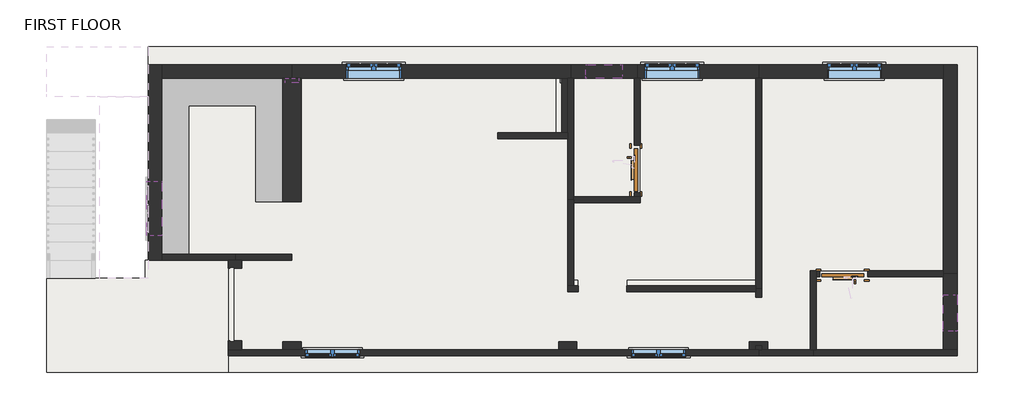
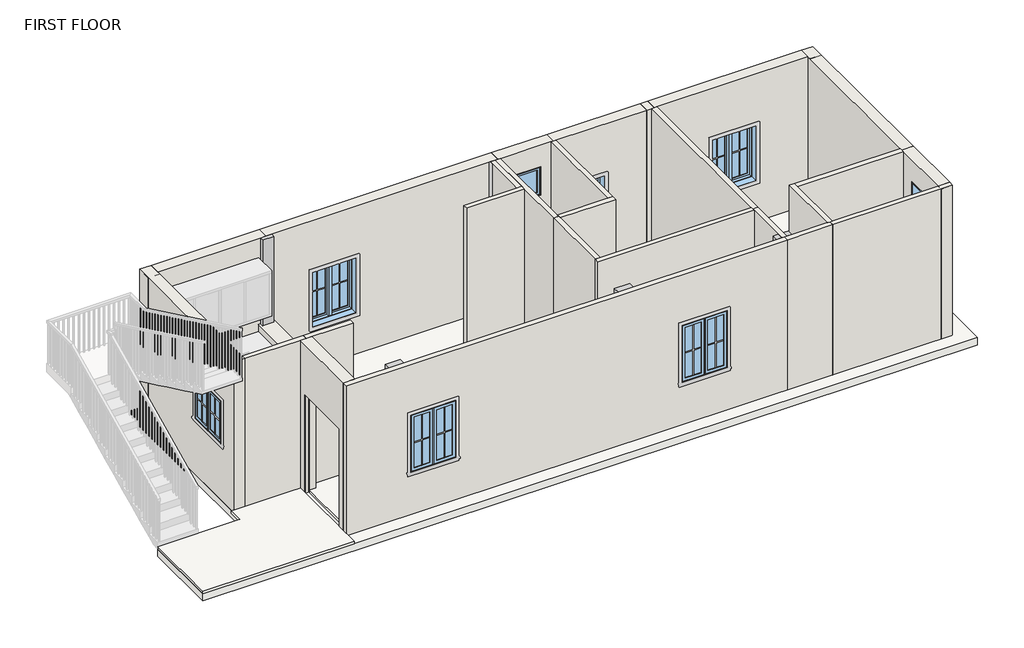
# One storey, part 1 of 3: 26 walls, 8 windows, 6 columns, 4 slabs, 2 doors.
"""IFC4 building model written with IfcOpenShell, lengths in millimetres."""

from ifc_helpers import new_model, si_unit, frame, origin, place, context, project, spatial, polyline, outline, extrude, faceted_brep, transform, mapped, element, save
from components import apartment_toilet_door_15897_d3_toilet_d7560075, apartment_toilet_door_15897_d3_toilet_03746f18, window_80340324, window_casement_double_w1_d341e8ac, window_casement_double_w1_80f1179f, window_casement_double_w1_2_90de19e9

model = new_model("IFC4")

# Units and contexts
model_context = context("Model", 3, world=origin())
ifc_project = project(units=[si_unit("LENGTHUNIT", "METRE", prefix="MILLI")], contexts=[model_context])

# Site, building, storey
site = spatial("IfcSite", under=ifc_project)
building = spatial("IfcBuilding", under=site)
storey = spatial("IfcBuildingStorey", under=building, Name="FIRST FLOOR", Elevation=3200.4)

# Columns
placement = place(None, origin())
element("IfcColumn", 1, ObjectType="Rectangular Column : 9\" X 12\"", at=placement, inside=storey, context=model_context, shape_type="SweptSolid", body=[
    extrude(outline(polyline([(-2166.0591227, 4797.7642852), (-2394.6591227, 4797.7642852), (-2394.6591227, 4873.9642852), (-2280.3591227, 4873.9642852), (-2166.0591227, 4873.9642852), (-2166.0591227, 4797.7642852)])), frame((0.0, 0.0, 4572.0), z_axis=(0.0, 0.0, 1.0), x_axis=(1.0, 0.0, 0.0)), (0.0, 0.0, 1.0), 1828.8),
])
element("IfcColumn", 2, ObjectType="Rectangular Column : 9\" X 12\"", at=placement, inside=storey, context=model_context, shape_type="Brep", body=[
    faceted_brep([(-4693.3591227, 5102.5642852, 3200.4), (-4464.7591227, 5102.5642852, 3200.4), (-4464.7591227, 4873.9642852, 3200.4), (-4464.7591227, 4797.7642852, 3200.4), (-4693.3591227, 4797.7642852, 3200.4), (-4693.3591227, 5102.5642852, 6400.8), (-4464.7591227, 5102.5642852, 6400.8), (-4464.7591227, 4873.9642852, 6400.8), (-4464.7591227, 4797.7642852, 6400.8), (-4693.3591227, 4797.7642852, 6400.8)], [[[0, 1, 2, 3, 4]], [[5, 6, 1, 0]], [[6, 7, 8, 3, 2, 1]], [[8, 9, 4, 3]], [[9, 5, 0, 4]], [[5, 9, 8, 7, 6]]]),
])
element("IfcColumn", 3, ObjectType="Rectangular Column : 9\" X 12\"", at=placement, inside=storey, context=model_context, shape_type="Brep", body=[
    faceted_brep([(5390.4408773, 454.3642852, 3200.4), (5695.2408773, 454.3642852, 3200.4), (5695.2408773, 327.3642852, 3200.4), (5593.6408773, 327.3642852, 3200.4), (5593.6408773, 390.8642852, 3200.4), (5492.0408773, 390.8642852, 3200.4), (5492.0408773, 327.3642852, 3200.4), (5390.4408773, 327.3642852, 3200.4), (5695.2408773, 454.3642852, 6400.8), (5695.2408773, 327.3642852, 6400.8), (5390.4408773, 454.3642852, 6400.8), (5390.4408773, 327.3642852, 6400.8), (5492.0408773, 454.3642852, 6400.8), (5492.0408773, 454.3642852, 5334.0), (5593.6408773, 454.3642852, 5334.0), (5593.6408773, 454.3642852, 6400.8), (5593.6408773, 327.3642852, 6400.8), (5593.6408773, 390.8642852, 5334.0), (5492.0408773, 390.8642852, 5334.0), (5492.0408773, 327.3642852, 6400.8)], [[[0, 1, 2, 3, 4, 5, 6, 7]], [[1, 8, 9, 2]], [[10, 0, 7, 11]], [[1, 0, 10, 12, 13, 14, 15, 8]], [[8, 15, 16, 9]], [[17, 4, 3, 16, 15, 14]], [[5, 18, 13, 12, 19, 6]], [[4, 17, 18, 5]], [[18, 17, 14, 13]], [[7, 6, 19, 11]], [[12, 10, 11, 19]], [[3, 2, 9, 16]]]),
])
element("IfcColumn", 4, ObjectType="Rectangular Column : 9\" X 12\"", at=placement, inside=storey, context=model_context, shape_type="SweptSolid", body=[
    extrude(outline(polyline([(2190.0408773, 454.3642852), (2494.8408773, 454.3642852), (2494.8408773, 327.3642852), (2190.0408773, 327.3642852), (2190.0408773, 454.3642852)])), frame((0.0, 0.0, 3200.4), z_axis=(0.0, 0.0, 1.0), x_axis=(1.0, 0.0, 0.0)), (0.0, 0.0, 1.0), 3200.4),
])
element("IfcColumn", 5, ObjectType="Rectangular Column : 9\" X 12\"", at=placement, inside=storey, context=model_context, shape_type="SweptSolid", body=[
    extrude(outline(polyline([(-2432.7591227, 454.3642852), (-2127.9591227, 454.3642852), (-2127.9591227, 327.3642852), (-2432.7591227, 327.3642852), (-2432.7591227, 454.3642852)])), frame((0.0, 0.0, 3200.4), z_axis=(0.0, 0.0, 1.0), x_axis=(1.0, 0.0, 0.0)), (0.0, 0.0, 1.0), 3200.4),
])
element("IfcColumn", 6, ObjectType="Rectangular Column : 9\" X 12\"", at=placement, inside=storey, context=model_context, shape_type="Brep", body=[
    faceted_brep([(-4693.3591227, 2130.7642852, 3200.4), (-4464.7591227, 2130.7642852, 3200.4), (-4464.7591227, 1927.5642852, 3200.4), (-4464.7591227, 1825.9642852, 3200.4), (-4693.3591227, 1825.9642852, 3200.4), (-4693.3591227, 2130.7642852, 6400.8), (-4464.7591227, 2130.7642852, 6400.8), (-4464.7591227, 1927.5642852, 6400.8), (-4464.7591227, 1825.9642852, 6400.8), (-4693.3591227, 1825.9642852, 6400.8)], [[[0, 1, 2, 3, 4]], [[5, 6, 1, 0]], [[6, 7, 8, 3, 2, 1]], [[8, 9, 4, 3]], [[9, 5, 0, 4]], [[5, 9, 8, 7, 6]]]),
])

# Doors
apartment_toilet_door_15897_d3_toilet_shape = apartment_toilet_door_15897_d3_toilet_d7560075(model_context)
element("IfcDoor", 7, ObjectType="Apartment_Toilet_Door_15897 : D3 TOILET", at=placement, inside=storey, context=model_context, shape_type="MappedRepresentation", body=[
    mapped(apartment_toilet_door_15897_d3_toilet_shape, transform((6952.5408773, 1597.3642852, 3200.4), x_axis=(-1.0, 0.0, 0.0), y_axis=(0.0, -1.0, 0.0), z_axis=(0.0, 0.0, 1.0))),
])
apartment_toilet_door_15897_d3_toilet_2_shape = apartment_toilet_door_15897_d3_toilet_03746f18(model_context)
element("IfcDoor", 8, ObjectType="Apartment_Toilet_Door_15897 : D3 TOILET", at=placement, inside=storey, context=model_context, shape_type="MappedRepresentation", body=[
    mapped(apartment_toilet_door_15897_d3_toilet_2_shape, transform((3510.8408773, 3337.2642852, 3200.4), x_axis=(0.0, -1.0, 0.0), y_axis=(1.0, 0.0, 0.0), z_axis=(0.0, 0.0, 1.0))),
])

# Slabs
element("IfcSlab", 9, ObjectType="6\" SLAB", at=placement, inside=storey, context=model_context, shape_type="SweptSolid", body=[
    extrude(outline(polyline([(9213.1408773, 5407.3642852), (9213.1408773, 113.4304234), (9213.1408773, -53.6357148), (-6395.1591227, -53.6357148), (-6395.1591227, 1521.1642852), (-4693.3591227, 1521.1642852), (-4693.3591227, 5407.3642852), (9213.1408773, 5407.3642852)])), frame((0.0, 0.0, 3048.0), z_axis=(0.0, 0.0, 1.0), x_axis=(1.0, 0.0, 0.0)), (0.0, 0.0, 1.0), 152.4),
])
element("IfcSlab", 10, ObjectType="FLOORING", at=placement, inside=storey, context=model_context, shape_type="SweptSolid", body=[
    extrude(outline(polyline([(-4464.7591227, 1927.5642852), (-4464.7591227, 4873.9642852), (-2432.7591227, 4873.9642852), (-2432.7591227, 2803.8642852), (-2127.9591227, 2803.8642852), (-2127.9591227, 4873.9642852), (2139.2408773, 4873.9642852), (2139.2408773, 3959.5642852), (1174.0408773, 3959.5642852), (1174.0408773, 3857.9642852), (2342.4408773, 3857.9642852), (2342.4408773, 1394.1642852), (2520.2408773, 1394.1642852), (2520.2408773, 1495.7642852), (2444.0408773, 1495.7642852), (2444.0408773, 2791.1642852), (3561.6408773, 2791.1642852), (3561.6408773, 4873.9642852), (5492.0408773, 4873.9642852), (5492.0408773, 1495.7642852), (3409.2408773, 1495.7642852), (3333.0408773, 1495.7642852), (3333.0408773, 1394.1642852), (5492.0408773, 1394.1642852), (5492.0408773, 1203.6642852), (5593.6408773, 1203.6642852), (5593.6408773, 4873.9642852), (8641.6408773, 4873.9642852), (8641.6408773, 1648.1642852), (6406.4408773, 1648.1642852), (6406.4408773, 327.3642852), (5593.6408773, 327.3642852), (5593.6408773, 390.8642852), (5492.0408773, 390.8642852), (5492.0408773, 327.3642852), (-3118.5591227, 327.3642852), (-3118.5591227, 397.6642852), (-3250.1591227, 397.6642852), (-3250.1591227, 1769.2642852), (-3118.5591227, 1769.2642852), (-3118.5591227, 1825.9642852), (-2280.3591227, 1825.9642852), (-2280.3591227, 1927.5642852), (-4464.7591227, 1927.5642852)])), frame((0.0, 0.0, 3200.4), z_axis=(0.0, 0.0, 1.0), x_axis=(1.0, 0.0, 0.0)), (0.0, 0.0, 1.0), 50.8),
])
element("IfcSlab", 11, ObjectType="FLOORING OPEN AREA", at=placement, inside=storey, context=model_context, shape_type="SweptSolid", body=[
    extrude(outline(polyline([(-3347.1591227, -53.6357148), (-6395.1591227, -53.6357148), (-6395.1591227, 1521.1642852), (-4744.1591227, 1521.1642852), (-4744.1591227, 1825.9642852), (-3347.1591227, 1825.9642852), (-3347.1591227, -53.6357148)])), frame((0.0, 0.0, 3200.4), z_axis=(0.0, 0.0, 1.0), x_axis=(1.0, 0.0, 0.0)), (0.0, 0.0, 1.0), 50.8),
])
element("IfcSlab", 12, ObjectType="FLOORING TOILET", at=placement, inside=storey, context=model_context, shape_type="SweptSolid", body=[
    extrude(outline(polyline([(7371.5408773, 1546.5642852), (8641.6408773, 1546.5642852), (8641.6408773, 327.3642852), (6508.0408773, 327.3642852), (6508.0408773, 1546.5642852), (6571.5408773, 1546.5642852), (6571.5408773, 1648.1642852), (7371.5408773, 1648.1642852), (7371.5408773, 1546.5642852)])), frame((0.0, 0.0, 3200.4), z_axis=(0.0, 0.0, 1.0), x_axis=(1.0, 0.0, 0.0)), (0.0, 0.0, 1.0), 50.8),
    extrude(outline(polyline([(3460.0408773, 4873.9642852), (3460.0408773, 3756.2642852), (3561.6408773, 3756.2642852), (3561.6408773, 2956.2642852), (3460.0408773, 2956.2642852), (3460.0408773, 2892.7642852), (2444.0408773, 2892.7642852), (2444.0408773, 4873.9642852), (3460.0408773, 4873.9642852)])), frame((0.0, 0.0, 3200.4), z_axis=(0.0, 0.0, 1.0), x_axis=(1.0, 0.0, 0.0)), (0.0, 0.0, 1.0), 50.8),
])

# Walls
element("IfcWall", 13, at=placement, inside=storey, context=model_context, shape_type="Brep", body=[
    faceted_brep([(-2432.7591227, 4873.9642852, 3200.4), (-2432.7591227, 2803.8642852, 3200.4), (-2432.7591227, 2803.8642852, 4572.0), (-2432.7591227, 4873.9642852, 4572.0), (-2127.9591227, 4873.9642852, 3200.4), (-2127.9591227, 4873.9642852, 4572.0), (-2127.9591227, 2803.8642852, 4572.0), (-2127.9591227, 2803.8642852, 3200.4), (-2280.3591227, 4873.9642852, 3200.4), (-2166.0591227, 4873.9642852, 4572.0), (-2280.3591227, 4873.9642852, 4572.0), (-2394.6591227, 4873.9642852, 4572.0)], [[[0, 1, 2, 3]], [[4, 5, 6, 7]], [[1, 0, 8, 4, 7]], [[2, 1, 7, 6]], [[3, 2, 6, 5, 9, 10, 11]], [[0, 3, 11, 10, 9, 5, 4, 8]]]),
])
element("IfcWall", 14, ObjectType="4\" WALL", at=placement, inside=storey, context=model_context, shape_type="Brep", body=[
    faceted_brep([(8870.2408773, 327.3642852, 3200.4), (8641.6408773, 327.3642852, 3200.4), (6508.0408773, 327.3642852, 3200.4), (6457.2408773, 327.3642852, 3200.4), (6457.2408773, 327.3642852, 6400.8), (6508.0408773, 327.3642852, 6400.8), (8641.6408773, 327.3642852, 6400.8), (8870.2408773, 327.3642852, 6400.8), (8870.2408773, 225.7642852, 3200.4), (8870.2408773, 225.7642852, 6400.8), (6457.2408773, 225.7642852, 6400.8), (6457.2408773, 225.7642852, 3200.4)], [[[0, 1, 2, 3, 4, 5, 6, 7]], [[8, 9, 10, 11]], [[3, 2, 1, 0, 8, 11]], [[4, 3, 11, 10]], [[7, 6, 5, 4, 10, 9]], [[0, 7, 9, 8]]]),
])
element("IfcWall", 15, ObjectType="4\" WALL", at=placement, inside=storey, context=model_context, shape_type="Brep", body=[
    faceted_brep([(-2280.3591227, 1927.5642852, 3200.4), (-3232.8591227, 1927.5642852, 3200.4), (-3232.8591227, 1927.5642852, 6400.8), (-2280.3591227, 1927.5642852, 6400.8), (-2280.3591227, 1825.9642852, 3200.4), (-2280.3591227, 1825.9642852, 6400.8), (-3118.5591227, 1825.9642852, 6400.8), (-3232.8591227, 1825.9642852, 6400.8), (-3232.8591227, 1825.9642852, 3200.4), (-3118.5591227, 1825.9642852, 3200.4)], [[[0, 1, 2, 3]], [[4, 5, 6, 7, 8, 9]], [[1, 0, 4, 9, 8]], [[2, 1, 8, 7]], [[3, 2, 7, 6, 5]], [[0, 3, 5, 4]]]),
])
element("IfcWall", 16, ObjectType="4\" WALL", at=placement, inside=storey, context=model_context, shape_type="Brep", body=[
    faceted_brep([(5593.6408773, 1343.3642852, 3200.4), (5593.6408773, 1343.3642852, 6400.8), (5593.6408773, 454.3642852, 6400.8), (5593.6408773, 327.3642852, 6400.8), (5593.6408773, 327.3642852, 3200.4), (5593.6408773, 390.8642852, 3200.4), (5593.6408773, 390.8642852, 5334.0), (5593.6408773, 454.3642852, 5334.0), (5593.6408773, 1203.6642852, 5334.0), (5593.6408773, 1203.6642852, 3200.4), (5492.0408773, 1343.3642852, 6400.8), (5492.0408773, 1343.3642852, 3200.4), (5492.0408773, 1292.5642852, 3200.4), (5492.0408773, 1203.6642852, 3200.4), (5492.0408773, 1203.6642852, 5334.0), (5492.0408773, 454.3642852, 5334.0), (5492.0408773, 390.8642852, 5334.0), (5492.0408773, 390.8642852, 3200.4), (5492.0408773, 327.3642852, 3200.4), (5492.0408773, 327.3642852, 6400.8), (5492.0408773, 454.3642852, 6400.8), (5492.0408773, 1292.5642852, 6400.8), (5542.8408773, 327.3642852, 3200.4), (5542.8408773, 327.3642852, 6400.8)], [[[0, 1, 2, 3, 4, 5, 6, 7, 8, 9]], [[10, 11, 12, 13, 14, 15, 16, 17, 18, 19, 20, 21]], [[11, 0, 9, 13, 12]], [[4, 22, 18, 17, 5]], [[1, 0, 11, 10]], [[3, 2, 1, 10, 21, 20, 19, 23]], [[4, 3, 23, 19, 18, 22]], [[16, 6, 5, 17]], [[6, 16, 15, 14, 8, 7]], [[8, 14, 13, 9]]]),
])
element("IfcWall", 17, ObjectType="4\" WALL", at=placement, inside=storey, context=model_context, shape_type="Brep", body=[
    faceted_brep([(5492.0408773, 1394.1642852, 3200.4), (3333.0408773, 1394.1642852, 3200.4), (3333.0408773, 1394.1642852, 5334.0), (2520.2408773, 1394.1642852, 5334.0), (2520.2408773, 1394.1642852, 3200.4), (2444.0408773, 1394.1642852, 3200.4), (2342.4408773, 1394.1642852, 3200.4), (2342.4408773, 1394.1642852, 6400.8), (2444.0408773, 1394.1642852, 6400.8), (5492.0408773, 1394.1642852, 6400.8), (3333.0408773, 1292.5642852, 5334.0), (3333.0408773, 1292.5642852, 3200.4), (5492.0408773, 1292.5642852, 3200.4), (5492.0408773, 1292.5642852, 6400.8), (2342.4408773, 1292.5642852, 6400.8), (2342.4408773, 1292.5642852, 3200.4), (2520.2408773, 1292.5642852, 3200.4), (2520.2408773, 1292.5642852, 5334.0), (5492.0408773, 1343.3642852, 3200.4), (5492.0408773, 1343.3642852, 6400.8)], [[[0, 1, 2, 3, 4, 5, 6, 7, 8, 9]], [[10, 11, 12, 13, 14, 15, 16, 17]], [[16, 15, 6, 5, 4]], [[12, 11, 1, 0, 18]], [[9, 8, 7, 14, 13, 19]], [[0, 9, 19, 13, 12, 18]], [[7, 6, 15, 14]], [[2, 1, 11, 10]], [[3, 2, 10, 17]], [[4, 3, 17, 16]]]),
])
element("IfcWall", 18, ObjectType="4\" WALL", at=placement, inside=storey, context=model_context, shape_type="Brep", body=[
    faceted_brep([(2444.0408773, 1394.1642852, 3200.4), (2444.0408773, 2791.1642852, 3200.4), (2444.0408773, 2841.9642852, 3200.4), (2444.0408773, 2841.9642852, 6400.8), (2444.0408773, 2791.1642852, 6400.8), (2444.0408773, 1394.1642852, 6400.8), (2342.4408773, 1394.1642852, 3200.4), (2342.4408773, 1394.1642852, 6400.8), (2342.4408773, 2841.9642852, 6400.8), (2342.4408773, 2841.9642852, 3200.4)], [[[0, 1, 2, 3, 4, 5]], [[6, 7, 8, 9]], [[2, 1, 0, 6, 9]], [[3, 2, 9, 8]], [[5, 4, 3, 8, 7]], [[0, 5, 7, 6]]]),
])
element("IfcWall", 19, ObjectType="4\" WALL", at=placement, inside=storey, context=model_context, shape_type="Brep", body=[
    faceted_brep([(2342.4408773, 3959.5642852, 3200.4), (2240.8408773, 3959.5642852, 3200.4), (1174.0408773, 3959.5642852, 3200.4), (1174.0408773, 3959.5642852, 6400.8), (2240.8408773, 3959.5642852, 6400.8), (2342.4408773, 3959.5642852, 6400.8), (2342.4408773, 3857.9642852, 3200.4), (2342.4408773, 3857.9642852, 6400.8), (1174.0408773, 3857.9642852, 6400.8), (1174.0408773, 3857.9642852, 3200.4)], [[[0, 1, 2, 3, 4, 5]], [[6, 7, 8, 9]], [[2, 1, 0, 6, 9]], [[3, 2, 9, 8]], [[5, 4, 3, 8, 7]], [[0, 5, 7, 6]]]),
])
element("IfcWall", 20, ObjectType="4\" WALL", at=placement, inside=storey, context=model_context, shape_type="Brep", body=[
    faceted_brep([(6508.0408773, 327.3642852, 3200.4), (6508.0408773, 1546.5642852, 3200.4), (6508.0408773, 1648.1642852, 3200.4), (6508.0408773, 1648.1642852, 6400.8), (6508.0408773, 1546.5642852, 6400.8), (6508.0408773, 327.3642852, 6400.8), (6406.4408773, 327.3642852, 3200.4), (6406.4408773, 327.3642852, 6400.8), (6406.4408773, 1648.1642852, 6400.8), (6406.4408773, 1648.1642852, 3200.4), (6457.2408773, 327.3642852, 3200.4), (6457.2408773, 327.3642852, 6400.8)], [[[0, 1, 2, 3, 4, 5]], [[6, 7, 8, 9]], [[2, 1, 0, 10, 6, 9]], [[5, 4, 3, 8, 7, 11]], [[0, 5, 11, 7, 6, 10]], [[3, 2, 9, 8]]]),
])
element("IfcWall", 21, ObjectType="4\" WALL", at=placement, inside=storey, context=model_context, shape_type="Brep", body=[
    faceted_brep([(6508.0408773, 1546.5642852, 3200.4), (6571.5408773, 1546.5642852, 3200.4), (6571.5408773, 1546.5642852, 5334.0), (7371.5408773, 1546.5642852, 5334.0), (7371.5408773, 1546.5642852, 3200.4), (8641.6408773, 1546.5642852, 3200.4), (8641.6408773, 1546.5642852, 6400.8), (6508.0408773, 1546.5642852, 6400.8), (6571.5408773, 1648.1642852, 5334.0), (6571.5408773, 1648.1642852, 3200.4), (6508.0408773, 1648.1642852, 3200.4), (6508.0408773, 1648.1642852, 6400.8), (8641.6408773, 1648.1642852, 6400.8), (8641.6408773, 1648.1642852, 3200.4), (7371.5408773, 1648.1642852, 3200.4), (7371.5408773, 1648.1642852, 5334.0), (8641.6408773, 1597.3642852, 3200.4), (8641.6408773, 1597.3642852, 6400.8)], [[[0, 1, 2, 3, 4, 5, 6, 7]], [[8, 9, 10, 11, 12, 13, 14, 15]], [[14, 13, 16, 5, 4]], [[10, 9, 1, 0]], [[7, 6, 17, 12, 11]], [[0, 7, 11, 10]], [[6, 5, 16, 13, 12, 17]], [[2, 1, 9, 8]], [[3, 2, 8, 15]], [[4, 3, 15, 14]]]),
])
element("IfcWall", 22, ObjectType="4\" WALL", at=placement, inside=storey, context=model_context, shape_type="Brep", body=[
    faceted_brep([(2444.0408773, 2791.1642852, 3200.4), (3561.6408773, 2791.1642852, 3200.4), (3561.6408773, 2791.1642852, 6400.8), (2444.0408773, 2791.1642852, 6400.8), (2444.0408773, 2892.7642852, 3200.4), (2444.0408773, 2892.7642852, 6400.8), (3460.0408773, 2892.7642852, 6400.8), (3561.6408773, 2892.7642852, 6400.8), (3561.6408773, 2892.7642852, 3200.4), (3460.0408773, 2892.7642852, 3200.4), (2444.0408773, 2841.9642852, 3200.4), (2444.0408773, 2841.9642852, 6400.8)], [[[0, 1, 2, 3]], [[4, 5, 6, 7, 8, 9]], [[1, 0, 10, 4, 9, 8]], [[3, 2, 7, 6, 5, 11]], [[0, 3, 11, 5, 4, 10]], [[2, 1, 8, 7]]]),
])
element("IfcWall", 23, ObjectType="4\" WALL", at=placement, inside=storey, context=model_context, shape_type="Brep", body=[
    faceted_brep([(3561.6408773, 2892.7642852, 3200.4), (3561.6408773, 2956.2642852, 3200.4), (3561.6408773, 2956.2642852, 5334.0), (3561.6408773, 3756.2642852, 5334.0), (3561.6408773, 3756.2642852, 3200.4), (3561.6408773, 4873.9642852, 3200.4), (3561.6408773, 4873.9642852, 6400.8), (3561.6408773, 2892.7642852, 6400.8), (3460.0408773, 2956.2642852, 5334.0), (3460.0408773, 2956.2642852, 3200.4), (3460.0408773, 2892.7642852, 3200.4), (3460.0408773, 2892.7642852, 6400.8), (3460.0408773, 4873.9642852, 6400.8), (3460.0408773, 4873.9642852, 3200.4), (3460.0408773, 3756.2642852, 3200.4), (3460.0408773, 3756.2642852, 5334.0), (3510.8408773, 4873.9642852, 3200.4), (3510.8408773, 4873.9642852, 6400.8)], [[[0, 1, 2, 3, 4, 5, 6, 7]], [[8, 9, 10, 11, 12, 13, 14, 15]], [[14, 13, 16, 5, 4]], [[10, 9, 1, 0]], [[7, 6, 17, 12, 11]], [[0, 7, 11, 10]], [[6, 5, 16, 13, 12, 17]], [[2, 1, 9, 8]], [[3, 2, 8, 15]], [[4, 3, 15, 14]]]),
])
element("IfcWall", 24, ObjectType="4\" WALL", at=placement, inside=storey, context=model_context, shape_type="Brep", body=[
    faceted_brep([(2342.4408773, 3959.5642852, 3200.4), (2342.4408773, 4873.9642852, 3200.4), (2342.4408773, 4873.9642852, 6400.8), (2342.4408773, 3959.5642852, 6400.8), (2240.8408773, 3959.5642852, 3200.4), (2240.8408773, 3959.5642852, 6400.8), (2240.8408773, 4797.7642852, 6400.8), (2240.8408773, 4873.9642852, 6400.8), (2240.8408773, 4873.9642852, 3200.4), (2240.8408773, 4797.7642852, 3200.4)], [[[0, 1, 2, 3]], [[4, 5, 6, 7, 8, 9]], [[1, 0, 4, 9, 8]], [[3, 2, 7, 6, 5]], [[2, 1, 8, 7]], [[0, 3, 5, 4]]]),
])
element("IfcWall", 25, ObjectType="4\" WALL", at=placement, inside=storey, context=model_context, shape_type="Brep", body=[
    faceted_brep([(2444.0408773, 2841.9642852, 3200.4), (2444.0408773, 2892.7642852, 3200.4), (2444.0408773, 4873.9642852, 3200.4), (2444.0408773, 4873.9642852, 6400.8), (2444.0408773, 2892.7642852, 6400.8), (2444.0408773, 2841.9642852, 6400.8), (2342.4408773, 2841.9642852, 3200.4), (2342.4408773, 2841.9642852, 6400.8), (2342.4408773, 3857.9642852, 6400.8), (2342.4408773, 3959.5642852, 6400.8), (2342.4408773, 4873.9642852, 6400.8), (2342.4408773, 4873.9642852, 3200.4), (2342.4408773, 3959.5642852, 3200.4), (2342.4408773, 3857.9642852, 3200.4), (2393.2408773, 4873.9642852, 3200.4), (2393.2408773, 4873.9642852, 6400.8)], [[[0, 1, 2, 3, 4, 5]], [[6, 7, 8, 9, 10, 11, 12, 13]], [[2, 1, 0, 6, 13, 12, 11, 14]], [[5, 4, 3, 15, 10, 9, 8, 7]], [[0, 5, 7, 6]], [[3, 2, 14, 11, 10, 15]]]),
])
element("IfcWall", 26, ObjectType="4\" WALL", at=placement, inside=storey, context=model_context, shape_type="Brep", body=[
    faceted_brep([(-3232.8591227, 1927.5642852, 3200.4), (-4464.7591227, 1927.5642852, 3200.4), (-4464.7591227, 1927.5642852, 6400.8), (-3232.8591227, 1927.5642852, 6400.8), (-3232.8591227, 1825.9642852, 3200.4), (-3232.8591227, 1825.9642852, 6400.8), (-3347.1591227, 1825.9642852, 6400.8), (-4464.7591227, 1825.9642852, 6400.8), (-4464.7591227, 1825.9642852, 3200.4), (-3347.1591227, 1825.9642852, 3200.4)], [[[0, 1, 2, 3]], [[4, 5, 6, 7, 8, 9]], [[1, 0, 4, 9, 8]], [[3, 2, 7, 6, 5]], [[0, 3, 5, 4]], [[2, 1, 8, 7]]]),
])
element("IfcWall", 27, ObjectType="4\" WALL", at=placement, inside=storey, context=model_context, shape_type="Brep", body=[
    faceted_brep([(5593.6408773, 1343.3642852, 3200.4), (5593.6408773, 4873.9642852, 3200.4), (5593.6408773, 4873.9642852, 6400.8), (5593.6408773, 1343.3642852, 6400.8), (5492.0408773, 1343.3642852, 3200.4), (5492.0408773, 1343.3642852, 6400.8), (5492.0408773, 1394.1642852, 6400.8), (5492.0408773, 4873.9642852, 6400.8), (5492.0408773, 4873.9642852, 3200.4), (5492.0408773, 1394.1642852, 3200.4), (5542.8408773, 4873.9642852, 3200.4), (5542.8408773, 4873.9642852, 6400.8)], [[[0, 1, 2, 3]], [[4, 5, 6, 7, 8, 9]], [[1, 0, 4, 9, 8, 10]], [[3, 2, 11, 7, 6, 5]], [[0, 3, 5, 4]], [[2, 1, 10, 8, 7, 11]]]),
])
element("IfcWall", 28, ObjectType="4\" WALL", at=placement, inside=storey, context=model_context, shape_type="Brep", body=[
    faceted_brep([(5542.8408773, 327.3642852, 3200.4), (5492.0408773, 327.3642852, 3200.4), (5390.4408773, 327.3642852, 3200.4), (2494.8408773, 327.3642852, 3200.4), (2190.0408773, 327.3642852, 3200.4), (-2127.9591227, 327.3642852, 3200.4), (-2432.7591227, 327.3642852, 3200.4), (-3118.5591227, 327.3642852, 3200.4), (-3347.1591227, 327.3642852, 3200.4), (-3347.1591227, 327.3642852, 6400.8), (-3118.5591227, 327.3642852, 6400.8), (-2432.7591227, 327.3642852, 6400.8), (-2127.9591227, 327.3642852, 6400.8), (2190.0408773, 327.3642852, 6400.8), (2494.8408773, 327.3642852, 6400.8), (5390.4408773, 327.3642852, 6400.8), (5492.0408773, 327.3642852, 6400.8), (5542.8408773, 327.3642852, 6400.8), (3409.2408773, 327.3642852, 5334.0), (3409.2408773, 327.3642852, 4114.8), (4323.6408773, 327.3642852, 4114.8), (4323.6408773, 327.3642852, 5334.0), (-2058.1091227, 327.3642852, 5334.0), (-2058.1091227, 327.3642852, 4114.8), (-1143.7091227, 327.3642852, 4114.8), (-1143.7091227, 327.3642852, 5334.0), (-3347.1591227, 225.7642852, 3200.4), (5542.8408773, 225.7642852, 3200.4), (5542.8408773, 225.7642852, 6400.8), (-3347.1591227, 225.7642852, 6400.8), (3409.2408773, 225.7642852, 5334.0), (4323.6408773, 225.7642852, 5334.0), (4323.6408773, 225.7642852, 4114.8), (3409.2408773, 225.7642852, 4114.8), (-2058.1091227, 225.7642852, 4114.8), (-2058.1091227, 225.7642852, 5334.0), (-1143.7091227, 225.7642852, 5334.0), (-1143.7091227, 225.7642852, 4114.8)], [[[0, 1, 2, 3, 4, 5, 6, 7, 8, 9, 10, 11, 12, 13, 14, 15, 16, 17], [18, 19, 20, 21], [22, 23, 24, 25]], [[26, 27, 28, 29], [30, 31, 32, 33], [34, 35, 36, 37]], [[8, 7, 6, 5, 4, 3, 2, 1, 0, 27, 26]], [[17, 16, 15, 14, 13, 12, 11, 10, 9, 29, 28]], [[0, 17, 28, 27]], [[9, 8, 26, 29]], [[18, 21, 31, 30]], [[21, 20, 32, 31]], [[20, 19, 33, 32]], [[19, 18, 30, 33]], [[22, 35, 34, 23]], [[23, 34, 37, 24]], [[24, 37, 36, 25]], [[35, 22, 25, 36]]]),
])
element("IfcWall", 29, ObjectType="4\" WALL", at=placement, inside=storey, context=model_context, shape_type="Brep", body=[
    faceted_brep([(6457.2408773, 327.3642852, 3200.4), (6406.4408773, 327.3642852, 3200.4), (5695.2408773, 327.3642852, 3200.4), (5593.6408773, 327.3642852, 3200.4), (5542.8408773, 327.3642852, 3200.4), (5542.8408773, 327.3642852, 6400.8), (5593.6408773, 327.3642852, 6400.8), (5695.2408773, 327.3642852, 6400.8), (6406.4408773, 327.3642852, 6400.8), (6457.2408773, 327.3642852, 6400.8), (6457.2408773, 225.7642852, 3200.4), (6457.2408773, 225.7642852, 6400.8), (5542.8408773, 225.7642852, 6400.8), (5542.8408773, 225.7642852, 3200.4)], [[[0, 1, 2, 3, 4, 5, 6, 7, 8, 9]], [[10, 11, 12, 13]], [[4, 3, 2, 1, 0, 10, 13]], [[5, 4, 13, 12]], [[9, 8, 7, 6, 5, 12, 11]], [[0, 9, 11, 10]]]),
])
element("IfcWall", 30, ObjectType="9\" WALL", at=placement, inside=storey, context=model_context, shape_type="Brep", body=[
    faceted_brep([(8641.6408773, 5102.5642852, 3200.4), (5542.8408773, 5102.5642852, 3200.4), (5542.8408773, 5102.5642852, 6400.8), (8641.6408773, 5102.5642852, 6400.8), (7606.5908773, 5102.5642852, 5334.0), (6692.1908773, 5102.5642852, 5334.0), (6692.1908773, 5102.5642852, 4114.8), (7606.5908773, 5102.5642852, 4114.8), (8641.6408773, 4873.9642852, 3200.4), (8641.6408773, 4873.9642852, 6400.8), (5593.6408773, 4873.9642852, 6400.8), (5542.8408773, 4873.9642852, 6400.8), (5542.8408773, 4873.9642852, 3200.4), (5593.6408773, 4873.9642852, 3200.4), (7606.5908773, 4873.9642852, 5334.0), (7606.5908773, 4873.9642852, 4114.8), (6692.1908773, 4873.9642852, 4114.8), (6692.1908773, 4873.9642852, 5334.0)], [[[0, 1, 2, 3], [4, 5, 6, 7]], [[8, 9, 10, 11, 12, 13], [14, 15, 16, 17]], [[1, 0, 8, 13, 12]], [[2, 1, 12, 11]], [[3, 2, 11, 10, 9]], [[0, 3, 9, 8]], [[15, 14, 4, 7]], [[16, 15, 7, 6]], [[17, 16, 6, 5]], [[14, 17, 5, 4]]]),
])
element("IfcWall", 31, ObjectType="9\" WALL", at=placement, inside=storey, context=model_context, shape_type="Brep", body=[
    faceted_brep([(8870.2408773, 327.3642852, 3200.4), (8870.2408773, 1597.3642852, 3200.4), (8870.2408773, 1597.3642852, 6400.8), (8870.2408773, 327.3642852, 6400.8), (8870.2408773, 632.1642852, 5943.6), (8870.2408773, 1241.7642852, 5943.6), (8870.2408773, 1241.7642852, 5334.0), (8870.2408773, 632.1642852, 5334.0), (8641.6408773, 327.3642852, 3200.4), (8641.6408773, 327.3642852, 6400.8), (8641.6408773, 1546.5642852, 6400.8), (8641.6408773, 1597.3642852, 6400.8), (8641.6408773, 1597.3642852, 3200.4), (8641.6408773, 1546.5642852, 3200.4), (8641.6408773, 632.1642852, 5943.6), (8641.6408773, 632.1642852, 5334.0), (8641.6408773, 1241.7642852, 5334.0), (8641.6408773, 1241.7642852, 5943.6)], [[[0, 1, 2, 3], [4, 5, 6, 7]], [[8, 9, 10, 11, 12, 13], [14, 15, 16, 17]], [[1, 0, 8, 13, 12]], [[2, 1, 12, 11]], [[3, 2, 11, 10, 9]], [[0, 3, 9, 8]], [[15, 14, 4, 7]], [[16, 15, 7, 6]], [[17, 16, 6, 5]], [[14, 17, 5, 4]]]),
])
element("IfcWall", 32, ObjectType="9\" WALL", at=placement, inside=storey, context=model_context, shape_type="Brep", body=[
    faceted_brep([(-4464.7591227, 1825.9642852, 3200.4), (-4464.7591227, 1927.5642852, 3200.4), (-4464.7591227, 4873.9642852, 3200.4), (-4464.7591227, 5102.5642852, 3200.4), (-4464.7591227, 5102.5642852, 6400.8), (-4464.7591227, 4873.9642852, 6400.8), (-4464.7591227, 1927.5642852, 6400.8), (-4464.7591227, 1825.9642852, 6400.8), (-4464.7591227, 3146.7642852, 5334.0), (-4464.7591227, 3146.7642852, 4419.6), (-4464.7591227, 2232.3642852, 4419.6), (-4464.7591227, 2232.3642852, 5334.0), (-4693.3591227, 1825.9642852, 3200.4), (-4693.3591227, 1825.9642852, 6400.8), (-4693.3591227, 5102.5642852, 6400.8), (-4693.3591227, 5102.5642852, 3200.4), (-4693.3591227, 3146.7642852, 5334.0), (-4693.3591227, 2232.3642852, 5334.0), (-4693.3591227, 2232.3642852, 4419.6), (-4693.3591227, 3146.7642852, 4419.6)], [[[0, 1, 2, 3, 4, 5, 6, 7], [8, 9, 10, 11]], [[12, 13, 14, 15], [16, 17, 18, 19]], [[3, 2, 1, 0, 12, 15]], [[7, 6, 5, 4, 14, 13]], [[4, 3, 15, 14]], [[0, 7, 13, 12]], [[9, 8, 16, 19]], [[10, 9, 19, 18]], [[11, 10, 18, 17]], [[8, 11, 17, 16]]]),
])
element("IfcWall", 33, ObjectType="9\" WALL", at=placement, inside=storey, context=model_context, shape_type="Brep", body=[
    faceted_brep([(-3118.5591227, 1825.9642852, 6400.8), (-3118.5591227, 327.3642852, 6400.8), (-3118.5591227, 327.3642852, 3200.4), (-3118.5591227, 473.8642852, 3200.4), (-3118.5591227, 473.8642852, 5334.0), (-3118.5591227, 1693.0642852, 5334.0), (-3118.5591227, 1693.0642852, 3200.4), (-3118.5591227, 1825.9642852, 3200.4), (-3347.1591227, 327.3642852, 6400.8), (-3347.1591227, 1825.9642852, 6400.8), (-3347.1591227, 1825.9642852, 3200.4), (-3347.1591227, 1693.0642852, 3200.4), (-3347.1591227, 1693.0642852, 5334.0), (-3347.1591227, 473.8642852, 5334.0), (-3347.1591227, 473.8642852, 3200.4), (-3347.1591227, 327.3642852, 3200.4), (-3327.1591227, 473.8642852, 3200.4), (-3327.1591227, 458.8642852, 3200.4), (-3250.1591227, 458.8642852, 3200.4), (-3250.1591227, 473.8642852, 3200.4), (-3232.8591227, 1825.9642852, 3200.4), (-3250.1591227, 1693.0642852, 3200.4), (-3250.1591227, 1708.0642852, 3200.4), (-3327.1591227, 1708.0642852, 3200.4), (-3327.1591227, 1693.0642852, 3200.4), (-3232.8591227, 1825.9642852, 6400.8), (-3327.1591227, 1693.0642852, 5334.0), (-3327.1591227, 473.8642852, 5334.0), (-3327.1591227, 1708.0642852, 5349.0), (-3327.1591227, 458.8642852, 5349.0), (-3250.1591227, 1708.0642852, 5349.0), (-3250.1591227, 1693.0642852, 5334.0), (-3250.1591227, 473.8642852, 5334.0), (-3250.1591227, 458.8642852, 5349.0)], [[[0, 1, 2, 3, 4, 5, 6, 7]], [[8, 9, 10, 11, 12, 13, 14, 15]], [[2, 15, 14, 16, 17, 18, 19, 3]], [[10, 20, 7, 6, 21, 22, 23, 24, 11]], [[1, 0, 25, 9, 8]], [[2, 1, 8, 15]], [[24, 26, 12, 11]], [[27, 16, 14, 13]], [[26, 27, 13, 12]], [[26, 24, 23, 28, 29, 17, 16, 27]], [[28, 23, 22, 30]], [[30, 22, 21, 31, 32, 19, 18, 33]], [[29, 28, 30, 33]], [[17, 29, 33, 18]], [[31, 21, 6, 5]], [[19, 32, 4, 3]], [[32, 31, 5, 4]], [[0, 7, 20, 10, 9, 25]]]),
])
element("IfcWall", 34, ObjectType="9\" WALL", at=placement, inside=storey, context=model_context, shape_type="Brep", body=[
    faceted_brep([(-2280.3591227, 5102.5642852, 6400.8), (-2280.3591227, 5102.5642852, 3200.4), (-4464.7591227, 5102.5642852, 3200.4), (-4464.7591227, 5102.5642852, 6400.8), (-2280.3591227, 4873.9642852, 3200.4), (-2280.3591227, 4873.9642852, 6400.8), (-2394.6591227, 4873.9642852, 6400.8), (-4464.7591227, 4873.9642852, 6400.8), (-4464.7591227, 4873.9642852, 3200.4), (-2432.7591227, 4873.9642852, 3200.4)], [[[0, 1, 2, 3]], [[4, 5, 6, 7, 8, 9]], [[2, 1, 4, 9, 8]], [[0, 3, 7, 6, 5]], [[3, 2, 8, 7]], [[0, 5, 4, 1]]]),
])
element("IfcWall", 35, ObjectType="9\" WALL", at=placement, inside=storey, context=model_context, shape_type="Brep", body=[
    faceted_brep([(2393.2408773, 5102.5642852, 3200.4), (-2280.3591227, 5102.5642852, 3200.4), (-2280.3591227, 5102.5642852, 6400.8), (2393.2408773, 5102.5642852, 6400.8), (-451.5591227, 5102.5642852, 5334.0), (-1365.9591227, 5102.5642852, 5334.0), (-1365.9591227, 5102.5642852, 4114.8), (-451.5591227, 5102.5642852, 4114.8), (2393.2408773, 4873.9642852, 3200.4), (2393.2408773, 4873.9642852, 6400.8), (2342.4408773, 4873.9642852, 6400.8), (2240.8408773, 4873.9642852, 6400.8), (2215.4408773, 4873.9642852, 6400.8), (-2166.0591227, 4873.9642852, 6400.8), (-2280.3591227, 4873.9642852, 6400.8), (-2280.3591227, 4873.9642852, 3200.4), (-2127.9591227, 4873.9642852, 3200.4), (2215.4408773, 4873.9642852, 3200.4), (2240.8408773, 4873.9642852, 3200.4), (2342.4408773, 4873.9642852, 3200.4), (-451.5591227, 4873.9642852, 5334.0), (-451.5591227, 4873.9642852, 4114.8), (-1365.9591227, 4873.9642852, 4114.8), (-1365.9591227, 4873.9642852, 5334.0)], [[[0, 1, 2, 3], [4, 5, 6, 7]], [[8, 9, 10, 11, 12, 13, 14, 15, 16, 17, 18, 19], [20, 21, 22, 23]], [[1, 0, 8, 19, 18, 17, 16, 15]], [[3, 2, 14, 13, 12, 11, 10, 9]], [[0, 3, 9, 8]], [[1, 15, 14, 2]], [[20, 23, 5, 4]], [[23, 22, 6, 5]], [[22, 21, 7, 6]], [[21, 20, 4, 7]]]),
])
element("IfcWall", 36, ObjectType="9\" WALL", at=placement, inside=storey, context=model_context, shape_type="Brep", body=[
    faceted_brep([(5542.8408773, 5102.5642852, 3200.4), (3510.8408773, 5102.5642852, 3200.4), (3510.8408773, 5102.5642852, 6400.8), (5542.8408773, 5102.5642852, 6400.8), (4552.2408773, 5102.5642852, 5334.0), (3637.8408773, 5102.5642852, 5334.0), (3637.8408773, 5102.5642852, 4114.8), (4552.2408773, 5102.5642852, 4114.8), (5542.8408773, 4873.9642852, 3200.4), (5542.8408773, 4873.9642852, 6400.8), (5492.0408773, 4873.9642852, 6400.8), (3561.6408773, 4873.9642852, 6400.8), (3510.8408773, 4873.9642852, 6400.8), (3510.8408773, 4873.9642852, 3200.4), (3561.6408773, 4873.9642852, 3200.4), (5492.0408773, 4873.9642852, 3200.4), (4552.2408773, 4873.9642852, 5334.0), (4552.2408773, 4873.9642852, 4114.8), (3637.8408773, 4873.9642852, 4114.8), (3637.8408773, 4873.9642852, 5334.0)], [[[0, 1, 2, 3], [4, 5, 6, 7]], [[8, 9, 10, 11, 12, 13, 14, 15], [16, 17, 18, 19]], [[1, 0, 8, 15, 14, 13]], [[2, 1, 13, 12]], [[3, 2, 12, 11, 10, 9]], [[0, 3, 9, 8]], [[16, 19, 5, 4]], [[19, 18, 6, 5]], [[18, 17, 7, 6]], [[17, 16, 4, 7]]]),
])
element("IfcWall", 37, ObjectType="9\" WALL", at=placement, inside=storey, context=model_context, shape_type="Brep", body=[
    faceted_brep([(8870.2408773, 1597.3642852, 3200.4), (8870.2408773, 5102.5642852, 3200.4), (8870.2408773, 5102.5642852, 6400.8), (8870.2408773, 1597.3642852, 6400.8), (8641.6408773, 1597.3642852, 3200.4), (8641.6408773, 1597.3642852, 6400.8), (8641.6408773, 1648.1642852, 6400.8), (8641.6408773, 4873.9642852, 6400.8), (8641.6408773, 5102.5642852, 6400.8), (8641.6408773, 5102.5642852, 3200.4), (8641.6408773, 4873.9642852, 3200.4), (8641.6408773, 1648.1642852, 3200.4)], [[[0, 1, 2, 3]], [[4, 5, 6, 7, 8, 9, 10, 11]], [[1, 0, 4, 11, 10, 9]], [[3, 2, 8, 7, 6, 5]], [[0, 3, 5, 4]], [[2, 1, 9, 8]]]),
])
element("IfcWall", 38, ObjectType="9\" WALL", at=placement, inside=storey, context=model_context, shape_type="Brep", body=[
    faceted_brep([(3510.8408773, 5102.5642852, 3200.4), (2393.2408773, 5102.5642852, 3200.4), (2393.2408773, 5102.5642852, 6400.8), (3510.8408773, 5102.5642852, 6400.8), (2647.2408773, 5102.5642852, 5943.6), (2647.2408773, 5102.5642852, 5334.0), (3256.8408773, 5102.5642852, 5334.0), (3256.8408773, 5102.5642852, 5943.6), (3510.8408773, 4873.9642852, 3200.4), (3510.8408773, 4873.9642852, 6400.8), (3460.0408773, 4873.9642852, 6400.8), (2444.0408773, 4873.9642852, 6400.8), (2393.2408773, 4873.9642852, 6400.8), (2393.2408773, 4873.9642852, 3200.4), (2444.0408773, 4873.9642852, 3200.4), (3460.0408773, 4873.9642852, 3200.4), (2647.2408773, 4873.9642852, 5943.6), (3256.8408773, 4873.9642852, 5943.6), (3256.8408773, 4873.9642852, 5334.0), (2647.2408773, 4873.9642852, 5334.0)], [[[0, 1, 2, 3], [4, 5, 6, 7]], [[8, 9, 10, 11, 12, 13, 14, 15], [16, 17, 18, 19]], [[1, 0, 8, 15, 14, 13]], [[2, 1, 13, 12]], [[3, 2, 12, 11, 10, 9]], [[0, 3, 9, 8]], [[4, 7, 17, 16]], [[7, 6, 18, 17]], [[6, 5, 19, 18]], [[5, 4, 16, 19]]]),
])

# Windows
window_shape = window_80340324(model_context)
element("IfcWindow", 39, ObjectType="Fixed : 24\" x 24\"", at=placement, inside=storey, context=model_context, shape_type="MappedRepresentation", body=[
    mapped(window_shape, transform((2913.9408773, 4988.2642852, 4419.6), x_axis=(-1.0, 0.0, 0.0), y_axis=(0.0, -1.0, 0.0), z_axis=(0.0, 0.0, 1.0))),
])
element("IfcWindow", 40, ObjectType="Fixed : 24\" x 24\"", at=placement, inside=storey, context=model_context, shape_type="MappedRepresentation", body=[
    mapped(window_shape, transform((8755.9408773, 898.8642852, 4419.6), x_axis=(0.0, -1.0, 0.0), y_axis=(1.0, 0.0, 0.0), z_axis=(0.0, 0.0, 1.0))),
])
window_casement_double_w1_shape = window_casement_double_w1_d341e8ac(model_context)
element("IfcWindow", 41, ObjectType="Window-Casement-Double : w1", at=placement, inside=storey, context=model_context, shape_type="MappedRepresentation", body=[
    mapped(window_casement_double_w1_shape, transform((-908.7591227, 4988.2642852, 3200.4), x_axis=(1.0, 0.0, 0.0), y_axis=(0.0, 1.0, 0.0), z_axis=(0.0, 0.0, 1.0))),
])
element("IfcWindow", 42, ObjectType="Window-Casement-Double : w1", at=placement, inside=storey, context=model_context, shape_type="MappedRepresentation", body=[
    mapped(window_casement_double_w1_shape, transform((4095.0408773, 4988.2642852, 3200.4), x_axis=(1.0, 0.0, 0.0), y_axis=(0.0, 1.0, 0.0), z_axis=(0.0, 0.0, 1.0))),
])
element("IfcWindow", 43, ObjectType="Window-Casement-Double : w1", at=placement, inside=storey, context=model_context, shape_type="MappedRepresentation", body=[
    mapped(window_casement_double_w1_shape, transform((7149.3908773, 4988.2642852, 3200.4), x_axis=(1.0, 0.0, 0.0), y_axis=(0.0, 1.0, 0.0), z_axis=(0.0, 0.0, 1.0))),
])
window_casement_double_w1_2_shape = window_casement_double_w1_80f1179f(model_context)
element("IfcWindow", 44, ObjectType="Window-Casement-Double : w1", at=placement, inside=storey, context=model_context, shape_type="MappedRepresentation", body=[
    mapped(window_casement_double_w1_2_shape, transform((3866.4408773, 276.5642852, 3200.4), x_axis=(-1.0, 0.0, 0.0), y_axis=(0.0, -1.0, 0.0), z_axis=(0.0, 0.0, 1.0))),
])
element("IfcWindow", 45, ObjectType="Window-Casement-Double : w1", at=placement, inside=storey, context=model_context, shape_type="MappedRepresentation", body=[
    mapped(window_casement_double_w1_2_shape, transform((-1600.9091227, 276.5642852, 3200.4), x_axis=(-1.0, 0.0, 0.0), y_axis=(0.0, -1.0, 0.0), z_axis=(0.0, 0.0, 1.0))),
])
window_casement_double_w1_2_2_shape = window_casement_double_w1_2_90de19e9(model_context)
element("IfcWindow", 46, ObjectType="Window-Casement-Double : w1 2", at=placement, inside=storey, context=model_context, shape_type="MappedRepresentation", body=[
    mapped(window_casement_double_w1_2_2_shape, transform((-4579.0591227, 2689.5642852, 3505.2), x_axis=(0.0, 1.0, 0.0), y_axis=(-1.0, 0.0, 0.0), z_axis=(0.0, 0.0, 1.0))),
])

save(model, "model.ifc")

# Revit data of these elements
# Type "Rectangular Column : 9\" X 12\""
#   Assembly Code = "B1010200"
#   Depth = 0' - 9"
#   Offset Base = 0' - 0"
#   Offset Top = 0' - 0"
#   Width = 1' - 0"
#   Material = none
# Type "Apartment_Toilet_Door_15897 : D3 TOILET"
#   Type Mark = "15"
#   Panel Type = ""
#   Location [instance default] = ""
#   Door Type = "Semi Solid Flushed Wooden Door Laminated on Boths Sides- Bathroom / Laundry"
#   Construction Type Id = "DOOR"
#   Analytic Construction = "Wooden"
#   Threshold Depth = 0' - 1.1811"
#   Thickness = 0' - 2.12598"
#   Thermal Resistance (R) = 2.58758 (h·ft²·°F)/BTU
#   Heat Transfer Coefficient (U) = 0.386456 BTU/(h·ft²·°F)
#   Height = 7' - 0"
#   Trim Projection Ext = 0' - 0.98425"
#   Trim Projection Int = 0' - 0.98425"
#   Width = 2' - 6"
#   Define Thermal Properties by = 1
#   Threshold Material = BEL-Threshold material-Marble
#   Visual Light Transmittance = 0
#   Solar Heat Gain Coefficient = 0
#   Function = (empty or 0)
#   Wall Closure = (empty or 0)
# Type "6\" SLAB"
#   Assembly Code = "B1010"
#   Function = 0
#   Layers, outside or top first: 0' - 6" "Concrete, Lightweight" (function 1)
# Type "FLOORING"
#   Assembly Code = "B1010"
#   Function = 0
#   Layers, outside or top first: 0' - 2" "FLOORING" (function 1)
# Type "FLOORING OPEN AREA"
#   Assembly Code = "B1010"
#   Function = 0
#   Layers, outside or top first: 0' - 2" "OPEN AREA TILE" (function 1)
# Type "FLOORING TOILET"
#   Assembly Code = "B1010"
#   Function = 0
#   Layers, outside or top first: 0' - 2" "toilet wash room" (function 1)
# Type
#   Assembly Code = "B2010"
#   Layers, outside or top first: 1' - 0" "Brick, Common" (function 1)
# Type "4\" WALL"
#   Assembly Code = "B2010"
#   Layers, outside or top first: 0' - 4" "Brick, Common" (function 1)
# Type "9\" WALL"
#   Assembly Code = "B2010"
#   Layers, outside or top first: 0' - 9" "Brick, Common" (function 1)
# Type "Fixed : 24\" x 24\""
#   Type Mark = "4"
#   Construction Type Id = "GSP4R"
#   Assembly Code = "B2020100"
#   Analytic Construction = "1/8 in Pilkington single glazing"
#   Visual Light Transmittance = 0.9
#   Solar Heat Gain Coefficient = 0.78
#   Heat Transfer Coefficient (U) = 0.6496 BTU/(h·ft²·°F)
#   Height = 2' - 0"
#   Default Sill Height = 3' - 0"
#   Width = 2' - 0"
#   Window Inset = 0' - 0 3/4"
#   Define Thermal Properties by = 1
#   Define Thermal Properties by = 1
#   Glass Pane Material = Glass
#   Sash Material = Sash
#   Wall Closure = (empty or 0)
# Type "Window-Casement-Double : w1"
#   Type Mark = "14"
#   Fire Rating = "0.5h"
#   Assembly Code = "B2020100"
#   Analytic Construction = "Double glazing - domestic"
#   Frame Extension [instance default] = 0' - 0 1/4"
#   Window Inset [instance default] = 0' - 0"
#   Wall Thickness [instance default] = 0' - 6"
#   Interior Wall Closure [instance default] = 0' - 2 1/4"
#   Half Width = 1' - 6"
#   Visual Light Transmittance = 0.81
#   Thermal Resistance (R) = 1.8146 (h·ft²·°F)/BTU
#   Solar Heat Gain Coefficient = 0.76
#   Rough Width = 3' - 0 1/2"
#   Rough Height = 4' - 0 1/2"
#   Height = 4' - 0"
#   Heat Transfer Coefficient (U) = 0.5511 BTU/(h·ft²·°F)
#   Exterior Wall Closure [instance default] = 0' - 1 1/4"
#   Extension Jamb [instance default] = 0' - 2 1/4"
#   Default Sill Height = 3' - 0"
#   Width = 3' - 0"
#   Define Thermal Properties by = 0
#   Muntin Visibility = yes
#   Interior Trim Visibility [instance default] = yes
#   Exterior Trim Visibility [instance default] = yes
#   Extension Jamb Visibility [instance default] = yes
#   Muntin Pattern = Muntin Pattern_2x2 : Muntin Pattern_2x2
#   Interior Trim = Trim-Window-Interior-Flat : Picture Frame
#   Interior Frame Material = Wood - Stained
#   Glass Panel Material = Glass
#   Exterior Trim = Trim-Window-Exterior-Flat : with Sill
#   Wall Closure = (empty or 0)
# Type "Window-Casement-Double : w1 2"
#   Type Mark = "18"
#   Fire Rating = "0.5h"
#   Assembly Code = "B2020100"
#   Analytic Construction = "Double glazing - domestic"
#   Frame Extension [instance default] = 0' - 0 1/4"
#   Window Inset [instance default] = 0' - 0"
#   Wall Thickness [instance default] = 0' - 6"
#   Interior Wall Closure [instance default] = 0' - 2 1/4"
#   Half Width = 1' - 6"
#   Visual Light Transmittance = 0.81
#   Thermal Resistance (R) = 1.8146 (h·ft²·°F)/BTU
#   Solar Heat Gain Coefficient = 0.76
#   Rough Width = 3' - 0 1/2"
#   Rough Height = 3' - 0 1/2"
#   Height = 3' - 0"
#   Heat Transfer Coefficient (U) = 0.5511 BTU/(h·ft²·°F)
#   Exterior Wall Closure [instance default] = 0' - 1 1/4"
#   Extension Jamb [instance default] = 0' - 2 1/4"
#   Default Sill Height = 3' - 0"
#   Width = 3' - 0"
#   Muntin Visibility = yes
#   Interior Trim Visibility [instance default] = yes
#   Exterior Trim Visibility [instance default] = yes
#   Extension Jamb Visibility [instance default] = yes
#   Muntin Pattern = Muntin Pattern_2x2 : Muntin Pattern_2x2
#   Interior Trim = Trim-Window-Interior-Flat : Picture Frame
#   Interior Frame Material = Wood - Stained
#   Glass Panel Material = Glass
#   Exterior Trim = Trim-Window-Exterior-Flat : with Sill
#   Wall Closure = (empty or 0)
# Element 1 (IfcColumn, "Rectangular Column : 9\" X 12\"")
#   Phase Created = New Construction
#   Materials on its faces: "green kitchen", "Brick, Common"
# Elements 2, 6 (IfcColumn, "Rectangular Column : 9\" X 12\"")
#   Phase Created = New Construction
#   Materials on its faces: "Brick, Common"
# Element 3 (IfcColumn, "Rectangular Column : 9\" X 12\"")
#   Phase Created = New Construction
#   Materials on its faces: "Brick, Common", "blue lite"
# Elements 4, 5 (IfcColumn, "Rectangular Column : 9\" X 12\"")
#   Phase Created = New Construction
#   Materials on its faces: "lite white", "Brick, Common"
# Elements 7, 8 (IfcDoor, "Apartment_Toilet_Door_15897 : D3 TOILET")
#   Location = ""
#   Phase Created = New Construction
#   Materials on its faces: "Default", "Metal - IR - Satin Chrome", "BEL-Threshold material-Marble", "BEL-Threshold material-Mortar"
# Element 9 (IfcSlab, "6\" SLAB")
#   Height Offset From Level = 0' - 0"
#   Phase Created = New Construction
#   Materials on its faces: "Concrete, Lightweight"
# Element 10 (IfcSlab, "FLOORING")
#   built-in parameter 1001955 = -1.5708 (stored number, unit not read)
#   Height Offset From Level = 0' - 2"
#   Phase Created = New Construction
#   Materials on its faces: "FLOORING"
# Element 11 (IfcSlab, "FLOORING OPEN AREA")
#   built-in parameter 1001955 = -1.5708 (stored number, unit not read)
#   Height Offset From Level = 0' - 2"
#   Phase Created = New Construction
#   Materials on its faces: "OPEN AREA TILE"
# Element 12 (IfcSlab, "FLOORING TOILET")
#   built-in parameter 1001955 = 3.14159 (stored number, unit not read)
#   Height Offset From Level = 0' - 2"
#   Phase Created = New Construction
#   Materials on its faces: "toilet wash room"
# Element 13 (IfcWall)
#   Top Offset = -6' - 0"
#   Base Offset = 0' - 0"
#   wall height = 4' - 6"
#   Phase Created = New Construction
#   Base Constraint = FIRST FLOOR
#   Top Constraint = SECOND FLOOR
#   Materials on its faces: "Brick, Common", "lite white"
# Element 14 (IfcWall, "4\" WALL")
#   Top Offset = 0' - 0"
#   Base Offset = 0' - 0"
#   wall height = 10' - 6"
#   Phase Created = New Construction
#   Base Constraint = FIRST FLOOR
#   Top Constraint = SECOND FLOOR
#   Materials on its faces: "Brick, Common", "TOILET TILE"
# Element 15 (IfcWall, "4\" WALL")
#   Top Offset = 0' - 0"
#   Base Offset = 0' - 0"
#   wall height = 10' - 6"
#   Phase Created = New Construction
#   Base Constraint = FIRST FLOOR
#   Top Constraint = SECOND FLOOR
#   Materials on its faces: "Brick, Common", "lite white", "green kitchen"
# Elements 16, 18 (IfcWall, "4\" WALL")
#   Top Offset = 0' - 0"
#   Base Offset = 0' - 0"
#   wall height = 10' - 6"
#   Phase Created = New Construction
#   Base Constraint = FIRST FLOOR
#   Top Constraint = SECOND FLOOR
#   Materials on its faces: "Brick, Common", "blue lite", "lite white"
# Element 17 (IfcWall, "4\" WALL")
#   Top Offset = 0' - 0"
#   Base Offset = 0' - 0"
#   wall height = 10' - 6"
#   Phase Created = New Construction
#   Base Constraint = FIRST FLOOR
#   Top Constraint = SECOND FLOOR
#   Materials on its faces: "Brick, Common", "lite white", "blue lite"
# Element 19 (IfcWall, "4\" WALL")
#   Top Offset = 0' - 0"
#   Base Offset = 0' - 0"
#   wall height = 10' - 6"
#   Phase Created = New Construction
#   Base Constraint = FIRST FLOOR
#   Top Constraint = SECOND FLOOR
#   Materials on its faces: "lite white", "Brick, Common"
# Elements 20, 22, 23 (IfcWall, "4\" WALL")
#   Top Offset = 0' - 0"
#   Base Offset = 0' - 0"
#   wall height = 10' - 6"
#   Phase Created = New Construction
#   Base Constraint = FIRST FLOOR
#   Top Constraint = SECOND FLOOR
#   Materials on its faces: "Brick, Common", "blue lite", "TOILET TILE"
# Element 21 (IfcWall, "4\" WALL")
#   Top Offset = 0' - 0"
#   Base Offset = 0' - 0"
#   wall height = 10' - 6"
#   Phase Created = New Construction
#   Base Constraint = FIRST FLOOR
#   Top Constraint = SECOND FLOOR
#   Materials on its faces: "Brick, Common", "TOILET TILE", "blue lite"
# Elements 24, 28 (IfcWall, "4\" WALL")
#   Top Offset = 0' - 0"
#   Base Offset = 0' - 0"
#   wall height = 10' - 6"
#   Phase Created = New Construction
#   Base Constraint = FIRST FLOOR
#   Top Constraint = SECOND FLOOR
#   Materials on its faces: "Brick, Common", "lite white"
# Element 25 (IfcWall, "4\" WALL")
#   Top Offset = 0' - 0"
#   Base Offset = 0' - 0"
#   wall height = 10' - 6"
#   Phase Created = New Construction
#   Base Constraint = FIRST FLOOR
#   Top Constraint = SECOND FLOOR
#   Materials on its faces: "Brick, Common", "TOILET TILE", "lite white"
# Element 26 (IfcWall, "4\" WALL")
#   Top Offset = 0' - 0"
#   Base Offset = 0' - 0"
#   wall height = 10' - 6"
#   Phase Created = New Construction
#   Base Constraint = FIRST FLOOR
#   Top Constraint = SECOND FLOOR
#   Materials on its faces: "Brick, Common", "green kitchen"
# Elements 27, 29 (IfcWall, "4\" WALL")
#   Top Offset = 0' - 0"
#   Base Offset = 0' - 0"
#   wall height = 10' - 6"
#   Phase Created = New Construction
#   Base Constraint = FIRST FLOOR
#   Top Constraint = SECOND FLOOR
#   Materials on its faces: "Brick, Common", "blue lite"
# Elements 30, 36, 37 (IfcWall, "9\" WALL")
#   Top Offset = 0' - 0"
#   Base Offset = 0' - 0"
#   wall height = 10' - 6"
#   Phase Created = New Construction
#   Base Constraint = FIRST FLOOR
#   Top Constraint = SECOND FLOOR
#   Materials on its faces: "Brick, Common"
# Elements 31, 38 (IfcWall, "9\" WALL")
#   Top Offset = 0' - 0"
#   Base Offset = 0' - 0"
#   wall height = 10' - 6"
#   Phase Created = New Construction
#   Base Constraint = FIRST FLOOR
#   Top Constraint = SECOND FLOOR
#   Materials on its faces: "Brick, Common", "TOILET TILE"
# Elements 32, 34 (IfcWall, "9\" WALL")
#   Top Offset = 0' - 0"
#   Base Offset = 0' - 0"
#   wall height = 10' - 6"
#   Phase Created = New Construction
#   Base Constraint = FIRST FLOOR
#   Top Constraint = SECOND FLOOR
#   Materials on its faces: "Brick, Common", "green kitchen"
# Elements 33, 35 (IfcWall, "9\" WALL")
#   Top Offset = 0' - 0"
#   Base Offset = 0' - 0"
#   wall height = 10' - 6"
#   Phase Created = New Construction
#   Base Constraint = FIRST FLOOR
#   Top Constraint = SECOND FLOOR
#   Materials on its faces: "Brick, Common", "lite white"
# Element 39 (IfcWindow, "Fixed : 24\" x 24\"")
#   Mark = "16"
#   Phase Created = New Construction
#   Materials on its faces: "Sash", "Glass"
# Element 40 (IfcWindow, "Fixed : 24\" x 24\"")
#   Mark = "17"
#   Phase Created = New Construction
#   Materials on its faces: "Sash", "Glass"
# Element 41 (IfcWindow, "Window-Casement-Double : w1")
#   Mark = "11"
#   Window Inset = 0' - 0"
#   Interior Wall Closure = 0' - 2 1/4"
#   Frame Extension = 0' - 0 1/4"
#   Exterior Wall Closure = 0' - 1 1/4"
#   Interior Trim Visibility = yes
#   Exterior Trim Visibility = yes
#   Phase Created = New Construction
#   Materials on its faces: "Wood - Stained", "Glass"
# Element 42 (IfcWindow, "Window-Casement-Double : w1")
#   Mark = "12"
#   Window Inset = 0' - 0"
#   Interior Wall Closure = 0' - 2 1/4"
#   Frame Extension = 0' - 0 1/4"
#   Exterior Wall Closure = 0' - 1 1/4"
#   Interior Trim Visibility = yes
#   Exterior Trim Visibility = yes
#   Phase Created = New Construction
#   Materials on its faces: "Wood - Stained", "Glass"
# Element 43 (IfcWindow, "Window-Casement-Double : w1")
#   Mark = "13"
#   Window Inset = 0' - 0"
#   Interior Wall Closure = 0' - 2 1/4"
#   Frame Extension = 0' - 0 1/4"
#   Exterior Wall Closure = 0' - 1 1/4"
#   Interior Trim Visibility = yes
#   Exterior Trim Visibility = yes
#   Phase Created = New Construction
#   Materials on its faces: "Wood - Stained", "Glass"
# Element 44 (IfcWindow, "Window-Casement-Double : w1")
#   Mark = "14"
#   Window Inset = 0' - 0"
#   Interior Wall Closure = 0' - 2 1/4"
#   Frame Extension = 0' - 0 1/4"
#   Exterior Wall Closure = 0' - 1 1/4"
#   Interior Trim Visibility = yes
#   Exterior Trim Visibility = yes
#   Phase Created = New Construction
#   Materials on its faces: "Wood - Stained", "Glass"
# Element 45 (IfcWindow, "Window-Casement-Double : w1")
#   Mark = "34"
#   Window Inset = 0' - 0"
#   Interior Wall Closure = 0' - 2 1/4"
#   Frame Extension = 0' - 0 1/4"
#   Exterior Wall Closure = 0' - 1 1/4"
#   Interior Trim Visibility = yes
#   Exterior Trim Visibility = yes
#   Phase Created = New Construction
#   Materials on its faces: "Wood - Stained", "Glass"
# Element 46 (IfcWindow, "Window-Casement-Double : w1 2")
#   Mark = "36"
#   Window Inset = 0' - 0"
#   Interior Wall Closure = 0' - 2 1/4"
#   Frame Extension = 0' - 0 1/4"
#   Exterior Wall Closure = 0' - 1 1/4"
#   Interior Trim Visibility = yes
#   Exterior Trim Visibility = yes
#   Phase Created = New Construction
#   Materials on its faces: "Wood - Stained", "Glass"
# Materials
#   "BEL-Threshold material-Marble": colour RGB 197 197 199, transparency 0, Cost = 0
#   "Concrete, Lightweight": class "Concrete", colour RGB 142 141 140, transparency 0, Description = "Lightweight concrete", Cost = 0
#   "FLOORING": class "Generic", colour RGB 233 236 239, transparency 0, Cost = 0
#   "OPEN AREA TILE": class "Generic", colour RGB 120 120 120, transparency 0, Cost = 0
#   "toilet wash room": class "Generic", colour RGB 120 120 120, transparency 0, Cost = 0
#   "Brick, Common": class "Masonry", colour RGB 170 98 104, transparency 0, Description = "Common brick", Cost = 0
#   "Glass": class "Glass", colour RGB 0 128 192, transparency 0.75, Description = "Soda Lime Glass", Cost = 0
#   "Sash": class "Wood", colour RGB 224 178 126, transparency 0, Cost = 0
#   "Wood - Stained": class "Wood", colour RGB 224 178 126, transparency 0, Cost = 0
#   "green kitchen": class "Generic", colour RGB 133 178 44, transparency 0, Cost = 0
#   "blue lite": class "Generic", colour RGB 205 221 234, transparency 0, Cost = 0
#   "lite white": class "Generic", colour RGB 120 120 120, transparency 0, Cost = 0
#   "Default": colour RGB 127 127 127, transparency 0, Cost = 0
#   "Metal - IR - Satin Chrome": colour RGB 244 244 244, transparency 0, Cost = 0
#   "BEL-Threshold material-Mortar": colour RGB 141 151 158, transparency 0, Cost = 0
#   "TOILET TILE": class "Generic", colour RGB 120 120 120, transparency 0, Cost = 0
